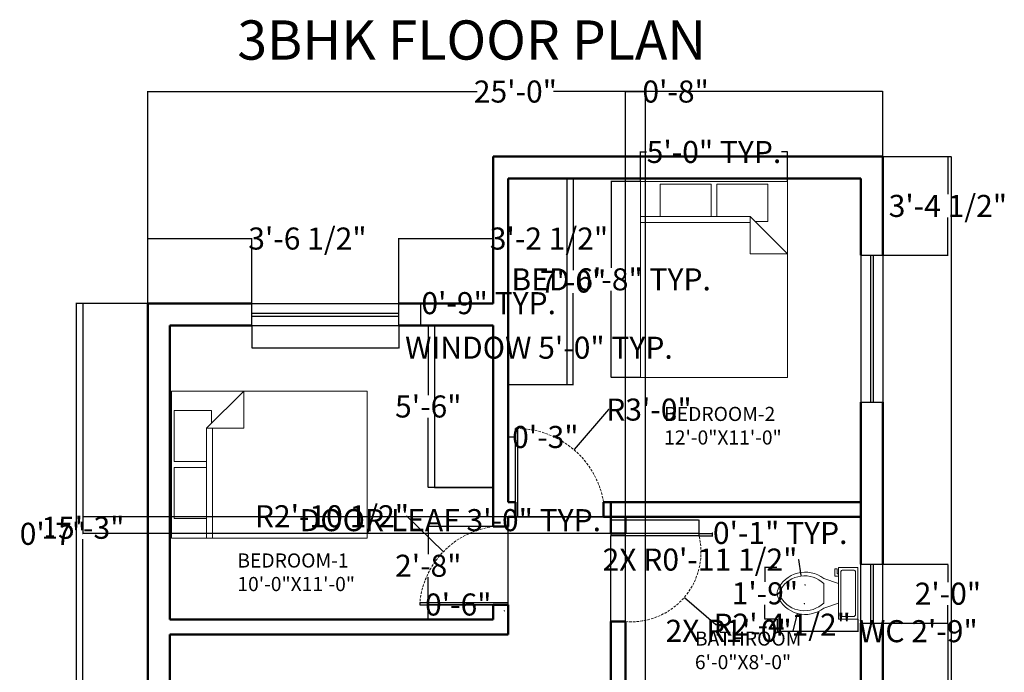
# Model space of a CAD drawing. Units: inches. Extents: x 4033 to 4435, y 499 to 1031.
# Tile 4 of 4: x 4033 to 4435, y 765 to 1031. Entities that reach past the tile are written whole.
import ezdxf

# ---------------------------------------------------------------- set-up
doc = ezdxf.new("R2010")
doc.units = ezdxf.units.IN
doc.header["$MEASUREMENT"] = 0
doc.linetypes.add('DASHEDX2', pattern=[1.5, 1, -0.5])
for name, color, linetype, lineweight in [('A-ANNO-DIMS', 2, 'Continuous', 18), ('A-ANNO-TEXT', 7, 'Continuous', 35), ('A-AREA-IDEN', 7, 'Continuous', 18), ('A-DOOR', 3, 'Continuous', 25), ('A-DOOR-SWNG', 3, 'DASHEDX2', 13), ('A-FLOR-CASE', 8, 'Continuous', 25), ('A-FLOR-FIXT', 8, 'Continuous', 18), ('A-FURN', 8, 'Continuous', 18), ('A-WALL', 7, 'Continuous', 50)]:
    doc.layers.add(name, color=color, linetype=linetype, lineweight=lineweight)
doc.layers.add('A-GLAZ', color=177, linetype='Continuous', lineweight=25, true_color=0x293189)
doc.styles.get("Standard").update_dxf_attribs({"font": 'arial.ttf'})
doc.dimstyles.get("Standard").update_dxf_attribs({"dimtxt": 9, "dimasz": 0.18, "dimexe": 0.18, "dimexo": 0.0625, "dimgap": 0.09, "dimtad": 0, "dimtih": 1, "dimtoh": 1, "dimdec": 0, "dimzin": 0, "dimdsep": 46, "dimlunit": 3, "dimtxsty": 'Standard', "dimcen": 0.09, "dimadec": 0, "dimazin": 0, "dimtfac": 1, "dimtdec": 0, "dimtofl": 0, "dimtmove": 0, "dimatfit": 3, "dimfxl": 1, "dimtolj": 1, "dimtzin": 0, "dimarcsym": 0})

# ---------------------------------------------------------------- blocks, each defined once
blk = doc.blocks.new('Bed - Queen')
for p, q in [((0, -80.00003), (0, 0)), ((0, 0), (59.99999, 0)), ((59.99999, 0), (59.99999, -80.00003)), ((7.99999, -1.2), (28.79998, -1.2)), ((7.99999, -14.4), (7.99999, -1.2)), ((28.79998, -1.2), (28.79998, -14.4)), ((31.19999, -1.2), (51.99999, -1.2)), ((31.19999, -14.4), (31.19999, -1.2)), ((51.99999, -1.2), (51.99999, -16.4)), ((0, -14.4), (44.8, -14.4)), ((59.99999, -29.6), (44.8, -14.4)), ((44.8, -14.4), (44.8, -29.6)), ((44.8, -16.8), (0, -16.8)), ((51.99999, -16.4), (46.79936, -16.4)), ((44.8, -29.6), (59.99999, -29.6)), ((59.99999, -80.00003), (0, -80.00003))]:
    blk.add_line(p, q)
blk = doc.blocks.new('Toilet - top')
for p, q in [((9.5, -6), (9.5, -2)), ((-8, -8.5), (-8, -8)), ((-7, -8), (-7, -9.5)), ((-4, -8), (-6, -14)), ((4, -8), (6, -14)), ((-10, -8.5), (-8, -8.5)), ((-10, -9.5), (-10, -8.5)), ((-7, -9.5), (-10, -9.5)), ((4, -14), (-4, -14))]:
    blk.add_line(p, q)
blk.add_lwpolyline([(10.5, -8), (10.5, 0), (-10.5, 0), (-10.5, -8)], close=True)
for points in [[(-9.5, -2), (-9.5, -6)], [(8.5, -1), (-8.5, -1)], [(-8.5, -7), (8.5, -7)]]:
    blk.add_lwpolyline(points)
for centre, radius, start, end in [((-8.62, -1.88), 0.884, 81.8699, 188.1301), ((8.62, -1.88), 0.884, 351.8699, 98.1301), ((-8.62, -6.12), 0.884, 171.8699, 278.1301), ((8.62, -6.12), 0.884, 261.8699, 8.1301), ((3.52, -21.58), 12.17, 141.4691, 247.9714), ((4.2, -21.82), 11.33, 136.3677, 238.9468), ((-3.52, -21.58), 12.17, 292.0284, 38.5307), ((-4.2, -21.82), 11.33, 301.053, 43.6321), ((0, -27.88), 4, 245.7318, 294.2682), ((0, -29), 4, 254.8605, 285.1395)]:
    blk.add_arc(centre, radius, start, end)
blk = doc.blocks.new('*D10')
at = {"layer": 'A-ANNO-DIMS', "color": 0, "lineweight": -2, "transparency": 16777216}
for p, q in [((4085.12, 915.25), (4055.73, 915.25)), ((4055.91, 915.07), (4055.91, 727.94)), ((4055.91, 531.43), (4055.91, 718.56)), ((4085.12, 531.25), (4055.73, 531.25))]:
    blk.add_line(p, q, dxfattribs=at)
at = {"layer": 'A-ANNO-DIMS', "color": 0, "transparency": 16777216}
for points in [[(4055.88, 915.07), (4055.94, 915.07), (4055.91, 915.25)], [(4055.88, 531.43), (4055.94, 531.43), (4055.91, 531.25)]]:
    blk.add_solid(points, dxfattribs=at)
at = {"layer": 'Defpoints', "color": 0, "transparency": 16777216}
for p in [(4055.91, 915.25), (4085.18, 915.25), (4085.18, 531.25)]:
    blk.add_point(p, dxfattribs=at)
at = {"layer": 'A-ANNO-DIMS', "color": 0, "transparency": 16777216, "insert": (4055.91, 723.25), "char_height": 9, "attachment_point": 5}
blk.add_mtext("\\A1;32'", dxfattribs=at)
blk = doc.blocks.new('*D11')
at = {"layer": 'A-ANNO-DIMS', "color": 0, "lineweight": -2, "transparency": 16777216}
for p, q in [((4305.74, 975.25), (4413.19, 975.25)), ((4413.01, 975.07), (4413.01, 757.94)), ((4413.01, 531.43), (4413.01, 748.56)), ((4349.24, 531.25), (4413.19, 531.25))]:
    blk.add_line(p, q, dxfattribs=at)
at = {"layer": 'A-ANNO-DIMS', "color": 0, "transparency": 16777216}
for points in [[(4412.98, 975.07), (4413.04, 975.07), (4413.01, 975.25)], [(4412.98, 531.43), (4413.04, 531.43), (4413.01, 531.25)]]:
    blk.add_solid(points, dxfattribs=at)
at = {"layer": 'Defpoints', "color": 0, "transparency": 16777216}
for p in [(4305.68, 975.25), (4413.01, 975.25), (4349.18, 531.25)]:
    blk.add_point(p, dxfattribs=at)
at = {"layer": 'A-ANNO-DIMS', "color": 0, "transparency": 16777216, "insert": (4413.01, 753.25), "char_height": 9, "attachment_point": 5}
blk.add_mtext("\\A1;37'", dxfattribs=at)
blk = doc.blocks.new('WIN-60IN')
for p, q in [((0, 0), (0, 9)), ((0, 9), (60, 9)), ((60, 0), (60, 9)), ((0, 5.1), (60, 5.1)), ((0, 3.9), (60, 3.9)), ((0, 0), (60, 0))]:
    blk.add_line(p, q)
blk = doc.blocks.new('DOOR-LEAF-36IN')
for p, q in [((0, 0), (0, 36)), ((1, 36), (0, 36)), ((1, 0), (1, 36)), ((0, 0), (1, 0))]:
    blk.add_line(p, q)
blk = doc.blocks.new('*D14')
at = {"layer": 'A-ANNO-DIMS', "color": 0, "lineweight": -2, "transparency": 16777216}
for p, q in [((4274.18, 826.86), (4274, 826.86)), ((4274.18, 821.52), (4274.18, 827.04)), ((4310, 826.86), (4274.36, 826.86)), ((4310.18, 821.52), (4310.18, 827.04))]:
    blk.add_line(p, q, dxfattribs=at)
at = {"layer": 'A-ANNO-DIMS', "color": 0, "transparency": 16777216}
for points in [[(4274.36, 826.89), (4274.36, 826.83), (4274.18, 826.86)], [(4310, 826.89), (4310, 826.83), (4310.18, 826.86)]]:
    blk.add_solid(points, dxfattribs=at)
at = {"layer": 'Defpoints', "color": 0, "transparency": 16777216}
for p in [(4274.18, 826.86), (4274.18, 821.46), (4310.18, 821.46)]:
    blk.add_point(p, dxfattribs=at)
at = {"layer": 'A-ANNO-DIMS', "color": 0, "transparency": 16777216, "insert": (4208.63, 826.86), "char_height": 9, "attachment_point": 5}
blk.add_mtext('\\A1;DOOR LEAF 3\'-0" TYP.', dxfattribs=at)
blk = doc.blocks.new('*D15')
at = {"layer": 'A-ANNO-DIMS', "color": 0, "lineweight": -2, "transparency": 16777216}
for p, q in [((4310.24, 821.46), (4315.76, 821.46)), ((4310.24, 820.46), (4315.76, 820.46)), ((4315.58, 821.46), (4315.58, 821.64)), ((4315.58, 821.64), (4315.76, 821.64)), ((4315.58, 820.64), (4315.58, 821.28))]:
    blk.add_line(p, q, dxfattribs=at)
at = {"layer": 'A-ANNO-DIMS', "color": 0, "transparency": 16777216}
for points in [[(4315.55, 821.28), (4315.61, 821.28), (4315.58, 821.46)], [(4315.55, 820.64), (4315.61, 820.64), (4315.58, 820.46)]]:
    blk.add_solid(points, dxfattribs=at)
at = {"layer": 'Defpoints', "color": 0, "transparency": 16777216}
for p in [(4310.18, 821.46), (4310.18, 820.46), (4315.58, 821.46)]:
    blk.add_point(p, dxfattribs=at)
at = {"layer": 'A-ANNO-DIMS', "color": 0, "transparency": 16777216, "insert": (4343.28, 821.64), "char_height": 9, "attachment_point": 5}
blk.add_mtext('\\A1;0\'-1" TYP.', dxfattribs=at)
blk = doc.blocks.new('*D16')
at = {"layer": 'A-ANNO-DIMS', "color": 0, "lineweight": -2, "transparency": 16777216}
for p, q in [((4127.58, 906.19), (4127.58, 897.07)), ((4187.58, 906.19), (4187.58, 897.07)), ((4127.76, 897.25), (4187.4, 897.25)), ((4187.58, 897.25), (4187.76, 897.25))]:
    blk.add_line(p, q, dxfattribs=at)
at = {"layer": 'A-ANNO-DIMS', "color": 0, "transparency": 16777216}
for points in [[(4127.76, 897.28), (4127.76, 897.22), (4127.58, 897.25)], [(4187.4, 897.28), (4187.4, 897.22), (4187.58, 897.25)]]:
    blk.add_solid(points, dxfattribs=at)
at = {"layer": 'Defpoints', "color": 0, "transparency": 16777216}
for p in [(4127.58, 906.25), (4187.58, 906.25), (4187.58, 897.25)]:
    blk.add_point(p, dxfattribs=at)
at = {"layer": 'A-ANNO-DIMS', "color": 0, "transparency": 16777216, "insert": (4244.79, 897.25), "char_height": 9, "attachment_point": 5}
blk.add_mtext('\\A1;WINDOW 5\'-0" TYP.', dxfattribs=at)
blk = doc.blocks.new('*D17')
at = {"layer": 'A-ANNO-DIMS', "color": 0, "lineweight": -2, "transparency": 16777216}
for p, q in [((4187.64, 915.25), (4196.76, 915.25)), ((4196.58, 915.25), (4196.58, 915.43)), ((4196.58, 915.43), (4196.76, 915.43)), ((4196.58, 906.43), (4196.58, 915.07)), ((4187.64, 906.25), (4196.76, 906.25))]:
    blk.add_line(p, q, dxfattribs=at)
at = {"layer": 'A-ANNO-DIMS', "color": 0, "transparency": 16777216}
for points in [[(4196.55, 915.07), (4196.61, 915.07), (4196.58, 915.25)], [(4196.55, 906.43), (4196.61, 906.43), (4196.58, 906.25)]]:
    blk.add_solid(points, dxfattribs=at)
at = {"layer": 'Defpoints', "color": 0, "transparency": 16777216}
for p in [(4187.58, 915.25), (4196.58, 915.25), (4187.58, 906.25)]:
    blk.add_point(p, dxfattribs=at)
at = {"layer": 'A-ANNO-DIMS', "color": 0, "transparency": 16777216, "insert": (4224.28, 915.43), "char_height": 9, "attachment_point": 5}
blk.add_mtext('\\A1;0\'-9" TYP.', dxfattribs=at)
blk = doc.blocks.new('*D18')
at = {"layer": 'A-ANNO-DIMS', "color": 0, "lineweight": -2, "transparency": 16777216}
for p, q in [((4286.2, 965.15), (4274.08, 965.15)), ((4274.26, 964.97), (4274.26, 929.83)), ((4274.26, 885.33), (4274.26, 920.46)), ((4286.2, 885.15), (4274.08, 885.15))]:
    blk.add_line(p, q, dxfattribs=at)
at = {"layer": 'A-ANNO-DIMS', "color": 0, "transparency": 16777216}
for points in [[(4274.23, 964.97), (4274.29, 964.97), (4274.26, 965.15)], [(4274.23, 885.33), (4274.29, 885.33), (4274.26, 885.15)]]:
    blk.add_solid(points, dxfattribs=at)
at = {"layer": 'Defpoints', "color": 0, "transparency": 16777216}
for p in [(4274.26, 965.15), (4286.26, 965.15), (4286.26, 885.15)]:
    blk.add_point(p, dxfattribs=at)
at = {"layer": 'A-ANNO-DIMS', "color": 0, "transparency": 16777216, "insert": (4274.26, 925.15), "char_height": 9, "attachment_point": 5}
blk.add_mtext('\\A1;BED 6\'-8" TYP.', dxfattribs=at)
blk = doc.blocks.new('*D19')
at = {"layer": 'A-ANNO-DIMS', "color": 0, "lineweight": -2, "transparency": 16777216}
for p, q in [((4286.26, 965.21), (4286.26, 977.33)), ((4286.44, 977.15), (4288.74, 977.15)), ((4346.08, 977.15), (4343.78, 977.15)), ((4346.26, 965.21), (4346.26, 977.33))]:
    blk.add_line(p, q, dxfattribs=at)
at = {"layer": 'A-ANNO-DIMS', "color": 0, "transparency": 16777216}
for points in [[(4286.44, 977.18), (4286.44, 977.12), (4286.26, 977.15)], [(4346.08, 977.18), (4346.08, 977.12), (4346.26, 977.15)]]:
    blk.add_solid(points, dxfattribs=at)
at = {"layer": 'Defpoints', "color": 0, "transparency": 16777216}
for p in [(4346.26, 977.15), (4286.26, 965.15), (4346.26, 965.15)]:
    blk.add_point(p, dxfattribs=at)
at = {"layer": 'A-ANNO-DIMS', "color": 0, "transparency": 16777216, "insert": (4316.26, 977.15), "char_height": 9, "attachment_point": 5}
blk.add_mtext('\\A1;5\'-0" TYP.', dxfattribs=at)
blk = doc.blocks.new('*D28')
at = {"layer": 'A-ANNO-DIMS', "color": 0, "lineweight": -2, "transparency": 16777216}
for p, q in [((4341.99, 786.44), (4341.99, 781.36)), ((4375.04, 786.44), (4375.04, 781.36)), ((4342.17, 781.54), (4374.86, 781.54)), ((4375.04, 781.54), (4375.22, 781.54))]:
    blk.add_line(p, q, dxfattribs=at)
at = {"layer": 'A-ANNO-DIMS', "color": 0, "transparency": 16777216}
for points in [[(4342.17, 781.57), (4342.17, 781.51), (4341.99, 781.54)], [(4374.86, 781.57), (4374.86, 781.51), (4375.04, 781.54)]]:
    blk.add_solid(points, dxfattribs=at)
at = {"layer": 'Defpoints', "color": 0, "transparency": 16777216}
for p in [(4341.99, 786.5), (4375.04, 786.5), (4375.04, 781.54)]:
    blk.add_point(p, dxfattribs=at)
at = {"layer": 'A-ANNO-DIMS', "color": 0, "transparency": 16777216, "insert": (4399.67, 781.54), "char_height": 9, "attachment_point": 5}
blk.add_mtext('\\A1;WC 2\'-9"', dxfattribs=at)
blk = doc.blocks.new('*D29')
at = {"layer": 'A-ANNO-DIMS', "color": 0, "lineweight": -2, "transparency": 16777216}
for p, q in [((4341.93, 807.5), (4336.86, 807.5)), ((4337.04, 807.32), (4337.04, 801.69)), ((4337.04, 786.68), (4337.04, 792.32)), ((4341.93, 786.5), (4336.86, 786.5))]:
    blk.add_line(p, q, dxfattribs=at)
at = {"layer": 'A-ANNO-DIMS', "color": 0, "transparency": 16777216}
for points in [[(4337.01, 807.32), (4337.07, 807.32), (4337.04, 807.5)], [(4337.01, 786.68), (4337.07, 786.68), (4337.04, 786.5)]]:
    blk.add_solid(points, dxfattribs=at)
at = {"layer": 'Defpoints', "color": 0, "transparency": 16777216}
for p in [(4341.99, 807.5), (4337.04, 786.5), (4341.99, 786.5)]:
    blk.add_point(p, dxfattribs=at)
at = {"layer": 'A-ANNO-DIMS', "color": 0, "transparency": 16777216, "insert": (4337.04, 797), "char_height": 9, "attachment_point": 5}
blk.add_mtext('\\A1;1\'-9"', dxfattribs=at)
blk = doc.blocks.new('*D32')
at = {"layer": 'A-ANNO-DIMS', "color": 0, "lineweight": -2, "transparency": 16777216}
for p, q in [((4085.18, 915.31), (4085.18, 1001.98)), ((4085.36, 1001.8), (4219.55, 1001.8)), ((4385, 1001.8), (4250.8, 1001.8)), ((4385.18, 975.31), (4385.18, 1001.98))]:
    blk.add_line(p, q, dxfattribs=at)
at = {"layer": 'A-ANNO-DIMS', "color": 0, "transparency": 16777216}
for points in [[(4085.36, 1001.83), (4085.36, 1001.77), (4085.18, 1001.8)], [(4385, 1001.83), (4385, 1001.77), (4385.18, 1001.8)]]:
    blk.add_solid(points, dxfattribs=at)
at = {"layer": 'Defpoints', "color": 0, "transparency": 16777216}
for p in [(4385.18, 1001.8), (4385.18, 975.25), (4085.18, 915.25)]:
    blk.add_point(p, dxfattribs=at)
at = {"layer": 'A-ANNO-DIMS', "color": 0, "transparency": 16777216, "insert": (4235.18, 1001.8), "char_height": 9, "attachment_point": 5}
blk.add_mtext('\\A1;25\'-0"', dxfattribs=at)
blk = doc.blocks.new('*D33')
at = {"layer": 'A-ANNO-DIMS', "color": 0, "lineweight": -2, "transparency": 16777216}
for p, q in [((4085.18, 915.31), (4085.18, 941.98)), ((4085.36, 941.8), (4127.4, 941.8)), ((4127.58, 915.31), (4127.58, 941.98)), ((4127.58, 941.8), (4127.76, 941.8))]:
    blk.add_line(p, q, dxfattribs=at)
at = {"layer": 'A-ANNO-DIMS', "color": 0, "transparency": 16777216}
for points in [[(4085.36, 941.83), (4085.36, 941.77), (4085.18, 941.8)], [(4127.4, 941.83), (4127.4, 941.77), (4127.58, 941.8)]]:
    blk.add_solid(points, dxfattribs=at)
at = {"layer": 'Defpoints', "color": 0, "transparency": 16777216}
for p in [(4127.58, 941.8), (4085.18, 915.25), (4127.58, 915.25)]:
    blk.add_point(p, dxfattribs=at)
at = {"layer": 'A-ANNO-DIMS', "color": 0, "transparency": 16777216, "insert": (4150.29, 941.8), "char_height": 9, "attachment_point": 5}
blk.add_mtext('\\A1;3\'-6 1/2"', dxfattribs=at)
blk = doc.blocks.new('*D34')
at = {"layer": 'A-ANNO-DIMS', "color": 0, "lineweight": -2, "transparency": 16777216}
for p, q in [((4187.58, 915.31), (4187.58, 941.98)), ((4187.76, 941.8), (4226, 941.8)), ((4226.18, 915.31), (4226.18, 941.98)), ((4226.18, 941.8), (4226.36, 941.8))]:
    blk.add_line(p, q, dxfattribs=at)
at = {"layer": 'A-ANNO-DIMS', "color": 0, "transparency": 16777216}
for points in [[(4187.76, 941.83), (4187.76, 941.77), (4187.58, 941.8)], [(4226, 941.83), (4226, 941.77), (4226.18, 941.8)]]:
    blk.add_solid(points, dxfattribs=at)
at = {"layer": 'Defpoints', "color": 0, "transparency": 16777216}
for p in [(4226.18, 941.8), (4187.58, 915.25), (4226.18, 915.25)]:
    blk.add_point(p, dxfattribs=at)
at = {"layer": 'A-ANNO-DIMS', "color": 0, "transparency": 16777216, "insert": (4248.89, 941.8), "char_height": 9, "attachment_point": 5}
blk.add_mtext('\\A1;3\'-2 1/2"', dxfattribs=at)
blk = doc.blocks.new('*D35')
at = {"layer": 'A-ANNO-DIMS', "color": 0, "lineweight": -2, "transparency": 16777216}
for p, q in [((4385.24, 975.25), (4411.91, 975.25)), ((4411.73, 975.07), (4411.73, 959.86)), ((4411.73, 935.16), (4411.73, 950.37)), ((4385.24, 934.98), (4411.91, 934.98))]:
    blk.add_line(p, q, dxfattribs=at)
at = {"layer": 'A-ANNO-DIMS', "color": 0, "transparency": 16777216}
for points in [[(4411.7, 975.07), (4411.76, 975.07), (4411.73, 975.25)], [(4411.7, 935.16), (4411.76, 935.16), (4411.73, 934.98)]]:
    blk.add_solid(points, dxfattribs=at)
at = {"layer": 'Defpoints', "color": 0, "transparency": 16777216}
for p in [(4385.18, 975.25), (4385.18, 934.98), (4411.73, 934.98)]:
    blk.add_point(p, dxfattribs=at)
at = {"layer": 'A-ANNO-DIMS', "color": 0, "transparency": 16777216, "insert": (4411.73, 955.12), "char_height": 9, "attachment_point": 5}
blk.add_mtext('\\A1;3\'-4 1/2"', dxfattribs=at)
blk = doc.blocks.new('*D38')
at = {"layer": 'A-ANNO-DIMS', "color": 0, "lineweight": -2, "transparency": 16777216}
for p, q in [((4085.12, 915.25), (4058.45, 915.25)), ((4058.63, 915.07), (4058.63, 828.44)), ((4058.63, 732.43), (4058.63, 819.06)), ((4085.12, 732.25), (4058.45, 732.25))]:
    blk.add_line(p, q, dxfattribs=at)
at = {"layer": 'A-ANNO-DIMS', "color": 0, "transparency": 16777216}
for points in [[(4058.6, 915.07), (4058.66, 915.07), (4058.63, 915.25)], [(4058.6, 732.43), (4058.66, 732.43), (4058.63, 732.25)]]:
    blk.add_solid(points, dxfattribs=at)
at = {"layer": 'Defpoints', "color": 0, "transparency": 16777216}
for p in [(4058.63, 915.25), (4085.18, 915.25), (4085.18, 732.25)]:
    blk.add_point(p, dxfattribs=at)
at = {"layer": 'A-ANNO-DIMS', "color": 0, "transparency": 16777216, "insert": (4058.63, 823.75), "char_height": 9, "attachment_point": 5}
blk.add_mtext('\\A1;15\'-3"', dxfattribs=at)
blk = doc.blocks.new('*D42')
at = {"layer": 'A-ANNO-DIMS', "color": 0, "lineweight": -2, "transparency": 16777216}
for p, q in [((4226.12, 792.25), (4199.45, 792.25)), ((4199.63, 792.25), (4199.63, 792.43)), ((4199.63, 792.43), (4199.81, 792.43)), ((4199.63, 786.43), (4199.63, 792.07)), ((4226.12, 786.25), (4199.45, 786.25))]:
    blk.add_line(p, q, dxfattribs=at)
at = {"layer": 'A-ANNO-DIMS', "color": 0, "transparency": 16777216}
for points in [[(4199.6, 792.07), (4199.66, 792.07), (4199.63, 792.25)], [(4199.6, 786.43), (4199.66, 786.43), (4199.63, 786.25)]]:
    blk.add_solid(points, dxfattribs=at)
at = {"layer": 'Defpoints', "color": 0, "transparency": 16777216}
for p in [(4199.63, 792.25), (4226.18, 792.25), (4226.18, 786.25)]:
    blk.add_point(p, dxfattribs=at)
at = {"layer": 'A-ANNO-DIMS', "color": 0, "transparency": 16777216, "insert": (4211.86, 792.43), "char_height": 9, "attachment_point": 5}
blk.add_mtext('\\A1;0\'-6"', dxfattribs=at)
blk = doc.blocks.new('*D43')
at = {"layer": 'A-ANNO-DIMS', "color": 0, "lineweight": -2, "transparency": 16777216}
for p, q in [((4226.12, 824.25), (4199.45, 824.25)), ((4199.63, 824.07), (4199.63, 812.94)), ((4199.63, 792.43), (4199.63, 803.56)), ((4226.12, 792.25), (4199.45, 792.25))]:
    blk.add_line(p, q, dxfattribs=at)
at = {"layer": 'A-ANNO-DIMS', "color": 0, "transparency": 16777216}
for points in [[(4199.6, 824.07), (4199.66, 824.07), (4199.63, 824.25)], [(4199.6, 792.43), (4199.66, 792.43), (4199.63, 792.25)]]:
    blk.add_solid(points, dxfattribs=at)
at = {"layer": 'Defpoints', "color": 0, "transparency": 16777216}
for p in [(4199.63, 824.25), (4226.18, 824.25), (4226.18, 792.25)]:
    blk.add_point(p, dxfattribs=at)
at = {"layer": 'A-ANNO-DIMS', "color": 0, "transparency": 16777216, "insert": (4199.63, 808.25), "char_height": 9, "attachment_point": 5}
blk.add_mtext('\\A1;2\'-8"', dxfattribs=at)
blk = doc.blocks.new('*D44')
at = {"layer": 'A-ANNO-DIMS', "color": 0, "lineweight": -2, "transparency": 16777216}
for p, q in [((4232.18, 834.31), (4232.18, 860.98)), ((4232.36, 860.8), (4235, 860.8)), ((4235.18, 834.31), (4235.18, 860.98)), ((4235.18, 860.8), (4235.36, 860.8))]:
    blk.add_line(p, q, dxfattribs=at)
at = {"layer": 'A-ANNO-DIMS', "color": 0, "transparency": 16777216}
for points in [[(4232.36, 860.83), (4232.36, 860.77), (4232.18, 860.8)], [(4235, 860.83), (4235, 860.77), (4235.18, 860.8)]]:
    blk.add_solid(points, dxfattribs=at)
at = {"layer": 'Defpoints', "color": 0, "transparency": 16777216}
for p in [(4235.18, 860.8), (4232.18, 834.25), (4235.18, 834.25)]:
    blk.add_point(p, dxfattribs=at)
at = {"layer": 'A-ANNO-DIMS', "color": 0, "transparency": 16777216, "insert": (4247.41, 860.8), "char_height": 9, "attachment_point": 5}
blk.add_mtext('\\A1;0\'-3"', dxfattribs=at)
blk = doc.blocks.new('*D48')
at = {"layer": 'A-ANNO-DIMS', "color": 0, "lineweight": -2, "transparency": 16777216}
for p, q in [((4226.12, 906.25), (4199.45, 906.25)), ((4199.63, 906.07), (4199.63, 877.94)), ((4199.63, 840.43), (4199.63, 868.56)), ((4226.12, 840.25), (4199.45, 840.25))]:
    blk.add_line(p, q, dxfattribs=at)
at = {"layer": 'A-ANNO-DIMS', "color": 0, "transparency": 16777216}
for points in [[(4199.6, 906.07), (4199.66, 906.07), (4199.63, 906.25)], [(4199.6, 840.43), (4199.66, 840.43), (4199.63, 840.25)]]:
    blk.add_solid(points, dxfattribs=at)
at = {"layer": 'Defpoints', "color": 0, "transparency": 16777216}
for p in [(4199.63, 906.25), (4226.18, 906.25), (4226.18, 840.25)]:
    blk.add_point(p, dxfattribs=at)
at = {"layer": 'A-ANNO-DIMS', "color": 0, "transparency": 16777216, "insert": (4199.63, 873.25), "char_height": 9, "attachment_point": 5}
blk.add_mtext('\\A1;5\'-6"', dxfattribs=at)
blk = doc.blocks.new('*D49')
at = {"layer": 'A-ANNO-DIMS', "color": 0, "lineweight": -2, "transparency": 16777216}
for p, q in [((4232.24, 966.25), (4258.91, 966.25)), ((4258.73, 966.07), (4258.73, 928.94)), ((4258.73, 882.43), (4258.73, 919.56)), ((4232.24, 882.25), (4258.91, 882.25))]:
    blk.add_line(p, q, dxfattribs=at)
at = {"layer": 'A-ANNO-DIMS', "color": 0, "transparency": 16777216}
for points in [[(4258.7, 966.07), (4258.76, 966.07), (4258.73, 966.25)], [(4258.7, 882.43), (4258.76, 882.43), (4258.73, 882.25)]]:
    blk.add_solid(points, dxfattribs=at)
at = {"layer": 'Defpoints', "color": 0, "transparency": 16777216}
for p in [(4232.18, 966.25), (4232.18, 882.25), (4258.73, 882.25)]:
    blk.add_point(p, dxfattribs=at)
at = {"layer": 'A-ANNO-DIMS', "color": 0, "transparency": 16777216, "insert": (4258.73, 924.25), "char_height": 9, "attachment_point": 5}
blk.add_mtext('\\A1;7\'-0"', dxfattribs=at)
blk = doc.blocks.new('*D51')
at = {"layer": 'A-ANNO-DIMS', "color": 0, "lineweight": -2, "transparency": 16777216}
for p, q in [((4385.24, 808.85), (4411.91, 808.85)), ((4411.73, 808.67), (4411.73, 801.54)), ((4411.73, 785.03), (4411.73, 792.17)), ((4385.24, 784.85), (4411.91, 784.85))]:
    blk.add_line(p, q, dxfattribs=at)
at = {"layer": 'A-ANNO-DIMS', "color": 0, "transparency": 16777216}
for points in [[(4411.7, 808.67), (4411.76, 808.67), (4411.73, 808.85)], [(4411.7, 785.03), (4411.76, 785.03), (4411.73, 784.85)]]:
    blk.add_solid(points, dxfattribs=at)
at = {"layer": 'Defpoints', "color": 0, "transparency": 16777216}
for p in [(4385.18, 808.85), (4411.73, 808.85), (4385.18, 784.85)]:
    blk.add_point(p, dxfattribs=at)
at = {"layer": 'A-ANNO-DIMS', "color": 0, "transparency": 16777216, "insert": (4411.73, 796.85), "char_height": 9, "attachment_point": 5}
blk.add_mtext('\\A1;2\'-0"', dxfattribs=at)
blk = doc.blocks.new('*D53')
at = {"layer": 'A-ANNO-DIMS', "color": 0, "lineweight": -2, "transparency": 16777216}
for p, q in [((4385.24, 784.85), (4411.91, 784.85)), ((4411.73, 784.67), (4411.73, 759.05)), ((4411.73, 724.05), (4411.73, 749.68)), ((4385.24, 723.87), (4411.91, 723.87))]:
    blk.add_line(p, q, dxfattribs=at)
at = {"layer": 'A-ANNO-DIMS', "color": 0, "transparency": 16777216}
for points in [[(4411.7, 784.67), (4411.76, 784.67), (4411.73, 784.85)], [(4411.7, 724.05), (4411.76, 724.05), (4411.73, 723.87)]]:
    blk.add_solid(points, dxfattribs=at)
at = {"layer": 'Defpoints', "color": 0, "transparency": 16777216}
for p in [(4385.18, 784.85), (4411.73, 784.85), (4385.18, 723.87)]:
    blk.add_point(p, dxfattribs=at)
at = {"layer": 'A-ANNO-DIMS', "color": 0, "transparency": 16777216, "insert": (4411.73, 754.36), "char_height": 9, "attachment_point": 5}
blk.add_mtext('\\A1;5\'-1"', dxfattribs=at)
blk = doc.blocks.new('*D57')
at = {"layer": 'A-ANNO-DIMS', "color": 0, "lineweight": -2, "transparency": 16777216}
for p, q in [((4280.12, 828.25), (4058.45, 828.25)), ((4058.63, 828.07), (4058.63, 821.64)), ((4280.12, 821.46), (4058.45, 821.46)), ((4058.63, 821.28), (4058.45, 821.28)), ((4058.63, 821.46), (4058.63, 821.28))]:
    blk.add_line(p, q, dxfattribs=at)
at = {"layer": 'A-ANNO-DIMS', "color": 0, "transparency": 16777216}
for points in [[(4058.6, 828.07), (4058.66, 828.07), (4058.63, 828.25)], [(4058.6, 821.64), (4058.66, 821.64), (4058.63, 821.46)]]:
    blk.add_solid(points, dxfattribs=at)
at = {"layer": 'Defpoints', "color": 0, "transparency": 16777216}
for p in [(4280.18, 828.25), (4058.63, 821.46), (4280.18, 821.46)]:
    blk.add_point(p, dxfattribs=at)
at = {"layer": 'A-ANNO-DIMS', "color": 0, "transparency": 16777216, "insert": (4046.4, 821.28), "char_height": 9, "attachment_point": 5}
blk.add_mtext('\\A1;0\'-7"', dxfattribs=at)
blk = doc.blocks.new('*D60')
at = {"layer": 'A-ANNO-DIMS', "color": 0, "lineweight": -2, "transparency": 16777216}
for p, q in [((4280.18, 750.31), (4280.18, 1001.98)), ((4280.36, 1001.8), (4288.18, 1001.8)), ((4288.36, 748.96), (4288.36, 1001.98)), ((4288.36, 1001.8), (4288.54, 1001.8))]:
    blk.add_line(p, q, dxfattribs=at)
at = {"layer": 'A-ANNO-DIMS', "color": 0, "transparency": 16777216}
for points in [[(4280.36, 1001.83), (4280.36, 1001.77), (4280.18, 1001.8)], [(4288.18, 1001.83), (4288.18, 1001.77), (4288.36, 1001.8)]]:
    blk.add_solid(points, dxfattribs=at)
at = {"layer": 'Defpoints', "color": 0, "transparency": 16777216}
for p in [(4288.36, 1001.8), (4280.18, 750.25), (4288.36, 748.89)]:
    blk.add_point(p, dxfattribs=at)
at = {"layer": 'A-ANNO-DIMS', "color": 0, "transparency": 16777216, "insert": (4300.59, 1001.8), "char_height": 9, "attachment_point": 5}
blk.add_mtext('\\A1;0\'-8"', dxfattribs=at)
blk = doc.blocks.new('*D63')
at = {"layer": 'A-ANNO-DIMS', "color": 0, "lineweight": -2, "transparency": 16777216}
for p, q in [((4273.17, 871.99), (4259.23, 855.72)), ((4273.35, 871.99), (4273.17, 871.99)), ((4235.59, 828.25), (4235.77, 828.25)), ((4235.68, 828.16), (4235.68, 828.34))]:
    blk.add_line(p, q, dxfattribs=at)
at = {"layer": 'A-ANNO-DIMS', "color": 0, "transparency": 16777216}
blk.add_solid([(4259.2, 855.74), (4259.25, 855.7), (4259.11, 855.59)], dxfattribs=at)
at = {"layer": 'Defpoints', "color": 0, "transparency": 16777216}
for p in [(4259.11, 855.59), (4235.68, 828.25)]:
    blk.add_point(p, dxfattribs=at)
at = {"layer": 'A-ANNO-DIMS', "color": 0, "transparency": 16777216, "insert": (4289.71, 871.99), "char_height": 9, "attachment_point": 5}
blk.add_mtext('\\A1;R3\'-0"', dxfattribs=at)
blk = doc.blocks.new('*D64')
at = {"layer": 'A-ANNO-DIMS', "color": 0, "lineweight": -2, "transparency": 16777216}
for p, q in [((4190.64, 828.45), (4190.82, 828.45)), ((4190.82, 828.45), (4205.64, 814.11)), ((4230.59, 789.88), (4230.77, 789.88)), ((4230.68, 789.79), (4230.68, 789.97))]:
    blk.add_line(p, q, dxfattribs=at)
at = {"layer": 'A-ANNO-DIMS', "color": 0, "transparency": 16777216}
blk.add_solid([(4205.66, 814.13), (4205.62, 814.09), (4205.77, 813.99)], dxfattribs=at)
at = {"layer": 'Defpoints', "color": 0, "transparency": 16777216}
for p in [(4205.77, 813.99), (4230.68, 789.88)]:
    blk.add_point(p, dxfattribs=at)
at = {"layer": 'A-ANNO-DIMS', "color": 0, "transparency": 16777216, "insert": (4160.3, 828.45), "char_height": 9, "attachment_point": 5}
blk.add_mtext('\\A1;R2\'-10 1/2"', dxfattribs=at)
blk = doc.blocks.new('*D66')
at = {"layer": 'A-ANNO-DIMS', "color": 0, "lineweight": -2, "transparency": 16777216}
for p, q in [((4282.36, 813.86), (4282.54, 813.86)), ((4282.45, 813.77), (4282.45, 813.95)), ((4317.07, 784.19), (4304.23, 795.2)), ((4317.25, 784.19), (4317.07, 784.19))]:
    blk.add_line(p, q, dxfattribs=at)
at = {"layer": 'A-ANNO-DIMS', "color": 0, "transparency": 16777216}
blk.add_solid([(4304.25, 795.22), (4304.21, 795.18), (4304.09, 795.32)], dxfattribs=at)
at = {"layer": 'Defpoints', "color": 0, "transparency": 16777216}
for p in [(4282.45, 813.86), (4304.09, 795.32)]:
    blk.add_point(p, dxfattribs=at)
at = {"layer": 'A-ANNO-DIMS', "color": 0, "transparency": 16777216, "insert": (4344.1, 784.19), "char_height": 9, "attachment_point": 5}
blk.add_mtext('\\A1;R2\'-4 1/2"', dxfattribs=at)
blk = doc.blocks.new('*D67')
at = {"layer": 'A-ANNO-DIMS', "color": 0, "lineweight": -2, "transparency": 16777216}
for p, q in [((4353.37, 800.52), (4353.55, 800.52)), ((4353.46, 800.43), (4353.46, 800.61)), ((4348.51, 781.69), (4350.32, 788.58)), ((4348.33, 781.69), (4348.51, 781.69))]:
    blk.add_line(p, q, dxfattribs=at)
at = {"layer": 'A-ANNO-DIMS', "color": 0, "transparency": 16777216}
blk.add_solid([(4350.29, 788.58), (4350.35, 788.57), (4350.37, 788.75)], dxfattribs=at)
at = {"layer": 'Defpoints', "color": 0, "transparency": 16777216}
for p in [(4353.46, 800.52), (4350.37, 788.75)]:
    blk.add_point(p, dxfattribs=at)
at = {"layer": 'A-ANNO-DIMS', "color": 0, "transparency": 16777216, "insert": (4322.23, 781.69), "char_height": 9, "attachment_point": 5}
blk.add_mtext('\\A1;2X R1\'-0"', dxfattribs=at)
blk = doc.blocks.new('*D68')
at = {"layer": 'A-ANNO-DIMS', "color": 0, "lineweight": -2, "transparency": 16777216}
for p, q in [((4350.63, 810.77), (4350.81, 810.77)), ((4350.81, 810.77), (4351.69, 804.21)), ((4353.13, 792.8), (4353.31, 792.8)), ((4353.22, 792.71), (4353.22, 792.89))]:
    blk.add_line(p, q, dxfattribs=at)
at = {"layer": 'A-ANNO-DIMS', "color": 0, "transparency": 16777216}
blk.add_solid([(4351.72, 804.21), (4351.66, 804.2), (4351.71, 804.03)], dxfattribs=at)
at = {"layer": 'Defpoints', "color": 0, "transparency": 16777216}
for p in [(4351.71, 804.03), (4353.22, 792.8)]:
    blk.add_point(p, dxfattribs=at)
at = {"layer": 'A-ANNO-DIMS', "color": 0, "transparency": 16777216, "insert": (4310.54, 810.77), "char_height": 9, "attachment_point": 5}
blk.add_mtext('\\A1;2X R0\'-11 1/2"', dxfattribs=at)

msp = doc.modelspace()

# ---------------------------------------------------------------- linework, layer by layer
at = {"layer": 'A-DOOR'}
for p, q in [((4236.18, 828.25), (4271.18, 828.25)), ((4232.18, 793.25), (4232.18, 824.25)), ((4274.18, 785.46), (4274.18, 820.46))]:
    msp.add_line(p, q, dxfattribs=at)
at = {"layer": 'A-DOOR-SWNG'}
for centre, radius, start, end in [((4235.68, 828.25), 36, 9.5931, 89.2043), ((4230.68, 789.88), 34.66, 97.459, 174.4194), ((4282.45, 813.86), 28.5, 265.4183, 13.3791)]:
    msp.add_arc(centre, radius, start, end, dxfattribs=at)
at = {"layer": 'A-FLOR-CASE'}
for p, q in [((4256.18, 966.25), (4256.18, 882.25)), ((4202.18, 906.25), (4202.18, 840.25)), ((4232.18, 882.25), (4256.18, 882.25)), ((4202.18, 840.25), (4226.18, 840.25))]:
    msp.add_line(p, q, dxfattribs=at)
at = {"layer": 'A-GLAZ'}
for p, q in [((4376.18, 808.85), (4385.18, 808.85)), ((4376.18, 784.85), (4376.18, 808.85)), ((4380.08, 808.85), (4380.08, 784.85)), ((4381.28, 808.85), (4381.28, 784.85)), ((4385.18, 784.85), (4385.18, 808.85)), ((4376.18, 784.85), (4385.18, 784.85))]:
    msp.add_line(p, q, dxfattribs=at)
at = {"layer": 'A-WALL'}
for p, q in [((4226.18, 975.25), (4226.18, 915.25)), ((4226.18, 975.25), (4385.18, 975.25)), ((4385.18, 975.25), (4385.18, 934.98)), ((4232.18, 966.25), (4232.18, 834.25)), ((4232.18, 966.25), (4376.18, 966.25)), ((4376.18, 966.25), (4376.18, 934.98)), ((4085.18, 915.25), (4127.58, 915.25)), ((4085.18, 915.25), (4085.18, 768.25)), ((4187.58, 915.25), (4226.18, 915.25)), ((4094.18, 906.25), (4127.58, 906.25)), ((4094.18, 906.25), (4094.18, 786.25)), ((4187.58, 906.25), (4226.18, 906.25)), ((4226.18, 906.25), (4226.18, 824.25)), ((4376.18, 874.98), (4376.18, 808.85)), ((4385.18, 874.98), (4385.18, 808.85)), ((4232.18, 834.25), (4235.18, 834.25)), ((4235.18, 834.25), (4235.18, 828.25)), ((4271.18, 834.25), (4271.18, 828.25)), ((4271.18, 834.25), (4376.18, 834.25)), ((4274.18, 834.25), (4274.18, 828.25)), ((4232.18, 828.25), (4235.18, 828.25)), ((4232.18, 828.25), (4232.18, 824.25)), ((4271.18, 828.25), (4376.18, 828.25)), ((4274.18, 828.25), (4274.18, 821.46)), ((4280.18, 828.25), (4280.18, 821.46)), ((4226.18, 824.25), (4232.18, 824.25)), ((4280.18, 821.46), (4274.18, 821.46)), ((4226.18, 792.25), (4232.18, 792.25)), ((4226.18, 792.25), (4226.18, 786.25)), ((4232.18, 792.25), (4232.18, 780.25)), ((4094.18, 786.25), (4226.18, 786.25)), ((4280.18, 785.46), (4274.18, 785.46)), ((4274.18, 785.46), (4274.18, 756.25)), ((4280.18, 785.46), (4280.18, 756.25)), ((4376.18, 784.85), (4376.18, 756.25)), ((4385.18, 784.85), (4385.18, 723.87)), ((4094.18, 780.25), (4094.18, 732.25)), ((4094.18, 780.25), (4232.18, 780.25)), ((4094.18, 780.25), (4094.18, 774.25)), ((4085.18, 768.25), (4085.18, 732.25))]:
    msp.add_line(p, q, dxfattribs=at)

# ---------------------------------------------------------------- block references
at = {"layer": 'A-DOOR'}
msp.add_blockref('DOOR-LEAF-36IN', (4235.18, 828.25), dxfattribs=at)
for p, rotation in [((4310.18, 820.46), 89.99999999999964), ((4196.18, 793.25), 270)]:
    msp.add_blockref('DOOR-LEAF-36IN', p, dxfattribs=dict(at, rotation=rotation))
at = {"layer": 'A-FLOR-FIXT', "rotation": 270}
msp.add_blockref('Toilet - top', (4375.04, 797), dxfattribs=at)
at = {"layer": 'A-FURN'}
msp.add_blockref('Bed - Queen', (4286.26, 965.15), dxfattribs=at)
at = {"layer": 'A-FURN', "rotation": 90}
msp.add_blockref('Bed - Queen', (4094.74, 819.57), dxfattribs=at)
at = {"layer": 'A-GLAZ', "rotation": 270.0000000000002}
msp.add_blockref('WIN-60IN', (4376.18, 934.98), dxfattribs=at)
at = {"layer": 'A-GLAZ'}
msp.add_blockref('WIN-60IN', (4127.58, 906.25), dxfattribs=at)

# ---------------------------------------------------------------- texts
at = {"layer": 'A-ANNO-TEXT', "insert": (4121.69, 1030.84), "char_height": 16.0203, "attachment_point": 1}
msp.add_mtext_dynamic_manual_height_columns('3BHK FLOOR PLAN ', width=308.3472, gutter_width=80.1, heights=[0], dxfattribs=at)
at = {"layer": 'A-AREA-IDEN', "char_height": 5.7683, "attachment_point": 1}
for s, width, insert in [('BEDROOM-2\\P12\'-0"X11\'-0"', 2.1401, (4295.89, 873.1)), ('BEDROOM-1\\P10\'-0"X11\'-0"', 5.7683, (4121.69, 813.28)), ('BATHROOM\\P6\'-0"X8\'-0"', 5.7683, (4308.46, 781.41))]:
    msp.add_mtext_dynamic_manual_height_columns(s, width=width, gutter_width=28.84, heights=[0], dxfattribs=dict(at, insert=insert))

# ---------------------------------------------------------------- dimensions: what is measured, and where the dimension line sits
at = {"layer": 'A-ANNO-DIMS'}
for base, p1, p2, picture, middle in [((4385.18, 1001.8), (4085.18, 915.25), (4385.18, 975.25), '*D32', (4235.18, 1001.8)), ((4288.36, 1001.8), (4280.18, 750.25), (4288.36, 748.89), '*D60', (4300.59, 1001.8)), ((4127.58, 941.8), (4085.18, 915.25), (4127.58, 915.25), '*D33', (4150.29, 941.8)), ((4226.18, 941.8), (4187.58, 915.25), (4226.18, 915.25), '*D34', (4248.89, 941.8)), ((4235.18, 860.8), (4232.18, 834.25), (4235.18, 834.25), '*D44', (4247.41, 860.8))]:
    dim = msp.add_linear_dim(base=base, p1=p1, p2=p2, dimstyle='Standard', override={"dimdec": 1, "dimlfac": 1, "dimrnd": 0, "dimzin": 1, "dimdsep": 46, "dimlunit": 4, "dimfrac": 2}, dxfattribs=at)
    dim.commit()
    dim.dimension.update_dxf_attribs({"geometry": picture, "text_midpoint": middle})
for base, p1, p2, text, picture, middle in [((4346.26, 977.15), (4286.26, 965.15), (4346.26, 965.15), '<> TYP.', '*D19', (4316.26, 977.15)), ((4187.58, 897.25), (4127.58, 906.25), (4187.58, 906.25), 'WINDOW <> TYP.', '*D16', (4244.79, 897.25)), ((4375.0386, 781.5442), (4341.9923, 786.5012), (4375.0386, 786.5012), 'WC <>', '*D28', (4399.6749, 781.5442))]:
    dim = msp.add_linear_dim(base=base, p1=p1, p2=p2, text=text, dimstyle='Standard', override={"dimdec": 1, "dimlfac": 1, "dimrnd": 0, "dimzin": 1, "dimdsep": 46, "dimlunit": 4, "dimfrac": 2}, dxfattribs=at)
    dim.commit()
    dim.dimension.update_dxf_attribs({"geometry": picture, "text_midpoint": middle})
for base, p1, p2, angle, override, picture, middle in [((4413.01, 975.25), (4349.18, 531.25), (4305.68, 975.25), 90, {"dimclrd": 0, "dimclre": 0, "dimclrt": 0}, '*D11', (4413.01, 753.25)), ((4411.73, 934.98), (4385.18, 975.25), (4385.18, 934.98), 270, {"dimdec": 1, "dimlfac": 1, "dimrnd": 0, "dimzin": 1, "dimdsep": 46, "dimlunit": 4, "dimfrac": 2}, '*D35', (4411.73, 955.12)), ((4258.73, 882.25), (4232.18, 966.25), (4232.18, 882.25), 270, {"dimdec": 1, "dimlfac": 1, "dimrnd": 0, "dimzin": 1, "dimdsep": 46, "dimlunit": 4, "dimfrac": 2}, '*D49', (4258.73, 924.25)), ((4058.63, 915.25), (4085.18, 732.25), (4085.18, 915.25), 90, {"dimdec": 1, "dimlfac": 1, "dimrnd": 0, "dimzin": 1, "dimdsep": 46, "dimlunit": 4, "dimfrac": 2}, '*D38', (4058.63, 823.75)), ((4055.91, 915.25), (4085.18, 531.25), (4085.18, 915.25), 90, {"dimclrd": 0, "dimclre": 0, "dimclrt": 0}, '*D10', (4055.91, 723.25)), ((4199.63, 906.25), (4226.18, 840.25), (4226.18, 906.25), 90, {"dimdec": 1, "dimlfac": 1, "dimrnd": 0, "dimzin": 1, "dimdsep": 46, "dimlunit": 4, "dimfrac": 2}, '*D48', (4199.63, 873.25)), ((4058.63, 821.46), (4280.18, 828.25), (4280.18, 821.46), 90, {"dimdec": 1, "dimlfac": 1, "dimrnd": 0, "dimzin": 1, "dimdsep": 46, "dimlunit": 4, "dimfrac": 2}, '*D57', (4046.4, 821.28)), ((4199.63, 824.25), (4226.18, 792.25), (4226.18, 824.25), 90, {"dimdec": 1, "dimlfac": 1, "dimrnd": 0, "dimzin": 1, "dimdsep": 46, "dimlunit": 4, "dimfrac": 2}, '*D43', (4199.63, 808.25)), ((4411.73, 808.85), (4385.18, 784.85), (4385.18, 808.85), 90, {"dimdec": 1, "dimlfac": 1, "dimrnd": 0, "dimzin": 1, "dimdsep": 46, "dimlunit": 4, "dimfrac": 2}, '*D51', (4411.73, 796.85)), ((4337.04, 786.5), (4341.99, 807.5), (4341.99, 786.5), 270, {"dimdec": 1, "dimlfac": 1, "dimrnd": 0, "dimzin": 1, "dimdsep": 46, "dimlunit": 4, "dimfrac": 2}, '*D29', (4337.04, 797)), ((4199.63, 792.25), (4226.18, 786.25), (4226.18, 792.25), 90, {"dimdec": 1, "dimlfac": 1, "dimrnd": 0, "dimzin": 1, "dimdsep": 46, "dimlunit": 4, "dimfrac": 2}, '*D42', (4211.86, 792.43)), ((4411.73, 784.85), (4385.18, 723.87), (4385.18, 784.85), 90, {"dimdec": 1, "dimlfac": 1, "dimrnd": 0, "dimzin": 1, "dimdsep": 46, "dimlunit": 4, "dimfrac": 2}, '*D53', (4411.73, 754.36))]:
    dim = msp.add_linear_dim(base=base, p1=p1, p2=p2, angle=angle, dimstyle='Standard', override=override, dxfattribs=at)
    dim.commit()
    dim.dimension.update_dxf_attribs({"geometry": picture, "text_midpoint": middle})
for base, p1, p2, angle, text, picture, middle in [((4274.26, 965.15), (4286.26, 885.15), (4286.26, 965.15), 90, 'BED <> TYP.', '*D18', (4274.26, 925.15)), ((4196.58, 915.25), (4187.58, 906.25), (4187.58, 915.25), 90, '<> TYP.', '*D17', (4224.28, 915.43)), ((4274.18, 826.86), (4310.18, 821.46), (4274.18, 821.46), 180, 'DOOR LEAF <> TYP.', '*D14', (4208.63, 826.86)), ((4315.58, 821.46), (4310.18, 820.46), (4310.18, 821.46), 90, '<> TYP.', '*D15', (4343.28, 821.64))]:
    dim = msp.add_linear_dim(base=base, p1=p1, p2=p2, angle=angle, text=text, dimstyle='Standard', override={"dimdec": 1, "dimlfac": 1, "dimrnd": 0, "dimzin": 1, "dimdsep": 46, "dimlunit": 4, "dimfrac": 2}, dxfattribs=at)
    dim.commit()
    dim.dimension.update_dxf_attribs({"geometry": picture, "text_midpoint": middle})
for center, mpoint, picture, middle in [((4235.68, 828.25), (4259.11, 855.59), '*D63', (4289.71, 871.99)), ((4230.68, 789.88), (4205.77, 813.99), '*D64', (4160.3, 828.45)), ((4282.45, 813.86), (4304.09, 795.32), '*D66', (4344.1, 784.19))]:
    dim = msp.add_radius_dim(center=center, mpoint=mpoint, dimstyle='Standard', override={"dimdec": 1, "dimlfac": 1, "dimrnd": 0, "dimzin": 1, "dimdsep": 46, "dimlunit": 4, "dimfrac": 2}, dxfattribs=at)
    dim.commit()
    dim.dimension.update_dxf_attribs({"geometry": picture, "text_midpoint": middle, "dimtype": 164})
for center, mpoint, picture, middle in [((4353.22, 792.8), (4351.71, 804.03), '*D68', (4310.54, 810.77)), ((4353.46, 800.52), (4350.37, 788.75), '*D67', (4322.23, 781.69))]:
    dim = msp.add_radius_dim(center=center, mpoint=mpoint, text='2X <>', dimstyle='Standard', override={"dimdec": 1, "dimlfac": 1, "dimrnd": 0, "dimzin": 1, "dimdsep": 46, "dimlunit": 4, "dimfrac": 2}, dxfattribs=at)
    dim.commit()
    dim.dimension.update_dxf_attribs({"geometry": picture, "text_midpoint": middle, "dimtype": 164})

doc.saveas('drawing.dxf')
